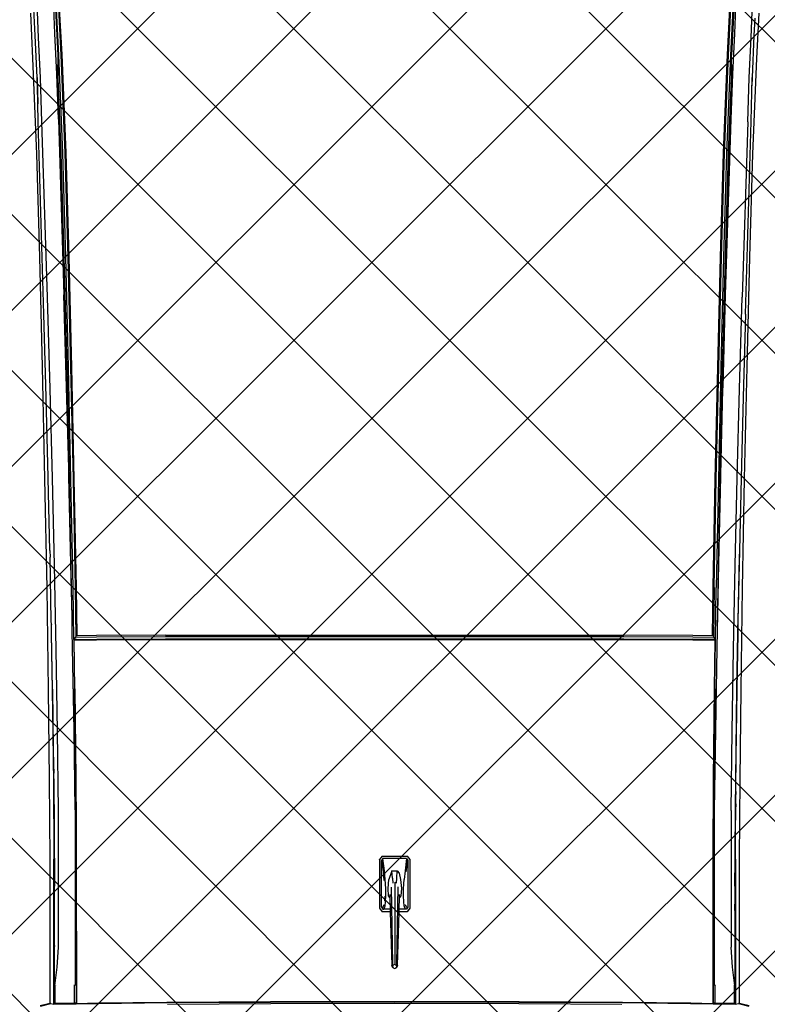
# Model space of a CAD drawing. Units: inches. Extents: x 2167 to 2589, y 1680 to 2489.
# Tile 16 of 38: x 2353 to 2387, y 1727 to 1772. Entities that reach past the tile are written whole.
import ezdxf

# ---------------------------------------------------------------- set-up
doc = ezdxf.new("R2010")
doc.units = ezdxf.units.IN
doc.header["$MEASUREMENT"] = 0
doc.layers.get('0').update_dxf_attribs({"color": 250})
doc.layers.add('C-PRKG-VEHS', color=8, linetype='Continuous', lineweight=13)
doc.layers.add('L-PVMT-PATT', color=252, linetype='Continuous', lineweight=13)
doc.layers.add('Edges', color=250, linetype='Continuous')

# ---------------------------------------------------------------- blocks, each defined once
blk = doc.blocks.new('Nissan Qashqai pl')
at = {"layer": 'Edges'}
for p, q in [((9.5168, 12.4903), (9.4761, 12.4919)), ((9.4782, 12.5024), (9.5503, 12.4987)), ((9.4862, 12.4961), (9.514, 12.4949)), ((9.514, 12.4949), (9.5811, 12.492)), ((9.5812, 12.4874), (9.5168, 12.4903)), ((9.5503, 12.4987), (9.7029, 12.4926)), ((9.651, 12.4906), (9.5811, 12.492)), ((9.5811, 12.492), (9.594, 12.4914)), ((9.6514, 12.4849), (9.5812, 12.4874)), ((9.9583, 12.4812), (9.651, 12.4906)), ((9.7029, 12.4926), (9.8673, 12.4878)), ((9.8673, 12.4878), (10.0423, 12.4835)), ((9.6514, 12.4849), (9.9312, 12.4761)), ((10.0776, 12.4719), (9.9312, 12.4761)), ((9.9583, 12.4812), (10.091, 12.4775)), ((10.0423, 12.4835), (10.2211, 12.4795)), ((10.2201, 12.4683), (10.0776, 12.4719)), ((10.091, 12.4775), (10.2202, 12.4743)), ((10.2202, 12.4743), (10.2203, 12.4743)), ((10.2203, 12.4743), (10.3353, 12.4717)), ((10.2211, 12.4795), (10.3955, 12.4762)), ((10.3353, 12.4717), (10.4477, 12.4694)), ((10.3353, 12.4717), (10.346, 12.4714)), ((10.3955, 12.4762), (10.5572, 12.4737)), ((10.5572, 12.4737), (10.7004, 12.4722)), ((10.7004, 12.4722), (10.8279, 12.4715)), ((11.0575, 12.4714), (11.0581, 12.4738)), ((11.0581, 12.4738), (11.0614, 12.4872)), ((11.0582, 12.47), (11.0624, 12.4866)), ((9.4694, 12.4654), (9.5105, 12.4637)), ((9.4706, 12.4561), (9.5443, 12.4522)), ((9.5446, 12.4542), (9.4709, 12.4581)), ((9.472, 12.463), (9.5454, 12.4591)), ((9.472, 12.4614), (9.5454, 12.4576)), ((9.5105, 12.4637), (9.5755, 12.4608)), ((9.5454, 12.4591), (9.5454, 12.4593)), ((9.5695, 12.4589), (9.5454, 12.4591)), ((9.5454, 12.4576), (9.7014, 12.4513)), ((9.5609, 12.4593), (9.5695, 12.4589)), ((9.5786, 12.4588), (9.5695, 12.4589)), ((9.5695, 12.4589), (9.7014, 12.4536)), ((9.5755, 12.4608), (9.6472, 12.4581)), ((9.6206, 12.4581), (9.5786, 12.4588)), ((9.6714, 12.4567), (9.6206, 12.4581)), ((9.6414, 12.458), (9.6407, 12.458)), ((9.6472, 12.4581), (9.9278, 12.4492)), ((9.6549, 12.4576), (9.6558, 12.4574)), ((9.6825, 12.4564), (9.6714, 12.4567)), ((9.6825, 12.4564), (9.6829, 12.4563)), ((9.6943, 12.456), (9.6825, 12.4564)), ((9.6943, 12.4558), (9.6943, 12.456)), ((9.6951, 12.456), (9.6943, 12.456)), ((9.6951, 12.4558), (9.6951, 12.456)), ((9.8565, 12.451), (9.6951, 12.456)), ((10.3586, 12.4651), (10.2201, 12.4683)), ((10.346, 12.4714), (10.4477, 12.4694)), ((10.4931, 12.4624), (10.3586, 12.4651)), ((10.4477, 12.4694), (10.4538, 12.4693)), ((10.4538, 12.4693), (10.4681, 12.469)), ((10.4676, 12.4691), (10.4538, 12.4693)), ((10.5566, 12.4677), (10.4676, 12.4691)), ((10.4676, 12.4691), (10.546, 12.4677)), ((10.4681, 12.469), (10.5866, 12.467)), ((10.6237, 12.4603), (10.4931, 12.4624)), ((10.546, 12.4677), (10.546, 12.4678)), ((10.546, 12.4677), (10.5576, 12.4675)), ((10.7, 12.4662), (10.5566, 12.4677)), ((10.5576, 12.4675), (10.6649, 12.4659)), ((10.5866, 12.467), (10.6649, 12.4659)), ((10.7502, 12.4586), (10.6237, 12.4603)), ((10.6649, 12.4659), (10.6786, 12.4658)), ((10.6649, 12.4659), (10.6772, 12.4657)), ((10.6786, 12.4657), (10.6772, 12.4657)), ((10.6786, 12.4658), (10.6786, 12.4662)), ((10.6786, 12.4657), (10.6786, 12.4658)), ((10.6786, 12.4658), (10.6801, 12.4657)), ((10.6786, 12.4657), (10.6801, 12.4657)), ((10.6801, 12.4662), (10.6801, 12.4657)), ((10.6801, 12.4657), (10.6801, 12.4657)), ((10.6801, 12.4657), (10.6811, 12.4657)), ((10.6801, 12.4657), (10.6811, 12.4657)), ((10.6811, 12.4662), (10.6811, 12.4657)), ((10.6811, 12.4657), (10.6811, 12.4657)), ((10.6811, 12.4657), (10.6966, 12.4654)), ((10.6811, 12.4657), (10.6991, 12.4655)), ((10.6811, 12.4657), (10.6991, 12.4655)), ((10.6966, 12.4654), (10.7144, 12.4653)), ((10.6991, 12.4655), (10.7144, 12.4653)), ((10.7201, 12.4661), (10.7, 12.4662)), ((10.7144, 12.4653), (10.7239, 12.4653)), ((10.7201, 12.4661), (10.7306, 12.4653)), ((10.7395, 12.4659), (10.7201, 12.4661)), ((10.7239, 12.4653), (10.7248, 12.4653)), ((10.7306, 12.4653), (10.7248, 12.4653)), ((10.7311, 12.4652), (10.7306, 12.4653)), ((10.7495, 12.4652), (10.7311, 12.4652)), ((10.7311, 12.4652), (10.7502, 12.4651)), ((10.7395, 12.4659), (10.7495, 12.4652)), ((10.7923, 12.4656), (10.7395, 12.4659)), ((10.8179, 12.4648), (10.7495, 12.4652)), ((10.7502, 12.4651), (10.7504, 12.4651)), ((10.7502, 12.4586), (10.968, 12.4585)), ((10.7504, 12.4651), (10.7808, 12.4649)), ((10.7808, 12.4649), (10.8179, 12.4648)), ((10.7923, 12.4652), (10.7923, 12.4656)), ((10.7933, 12.4656), (10.7923, 12.4656)), ((10.7933, 12.4652), (10.7933, 12.4656)), ((10.804, 12.4656), (10.7933, 12.4656)), ((10.804, 12.4653), (10.804, 12.4656)), ((10.8075, 12.4655), (10.804, 12.4656)), ((10.8075, 12.4655), (10.8075, 12.4653)), ((10.811, 12.4655), (10.8075, 12.4655)), ((10.811, 12.4655), (10.811, 12.4653)), ((10.8145, 12.4655), (10.811, 12.4655)), ((10.8145, 12.4653), (10.8145, 12.4655)), ((10.8279, 12.4654), (10.8145, 12.4655)), ((10.8277, 12.4647), (10.8179, 12.4648)), ((10.8711, 12.4646), (10.8277, 12.4647)), ((10.8279, 12.4715), (11.0544, 12.4714)), ((10.8279, 12.4654), (11.0592, 12.4653)), ((10.8711, 12.4646), (10.8824, 12.4646)), ((10.8824, 12.4646), (10.8825, 12.4646)), ((10.8825, 12.4646), (10.8884, 12.4646)), ((10.8884, 12.4646), (10.8923, 12.4646)), ((10.8923, 12.4646), (10.8996, 12.4646)), ((10.9097, 12.4646), (10.8996, 12.4646)), ((10.9097, 12.4646), (10.9399, 12.4646)), ((10.9399, 12.4646), (10.9491, 12.4645)), ((10.9491, 12.4645), (11.0301, 12.4645)), ((11, 12.4605), (10.968, 12.4585)), ((11.0301, 12.4645), (11, 12.4605)), ((11.0301, 12.4637), (11.0287, 12.4637)), ((11.03, 12.4635), (11.0301, 12.4637)), ((11.0301, 12.4642), (11.0301, 12.4645)), ((11.0574, 12.4637), (11.0301, 12.4637)), ((11.0544, 12.4714), (11.0575, 12.4714)), ((11.0568, 12.4323), (11.0574, 12.4637)), ((11.0574, 12.4637), (11.0592, 12.4653)), ((11.0575, 12.4714), (11.0582, 12.47)), ((11.0592, 12.4653), (11.0582, 12.47)), ((11.0585, 12.43), (11.0592, 12.4653)), ((9.5443, 12.4522), (9.701, 12.4459)), ((9.7011, 12.4478), (9.5446, 12.4542)), ((9.701, 12.4459), (9.8673, 12.441)), ((9.8673, 12.443), (9.7011, 12.4478)), ((9.7014, 12.4536), (9.8673, 12.4488)), ((9.7014, 12.4513), (9.8673, 12.4464)), ((9.9794, 12.4475), (9.8565, 12.451)), ((9.8673, 12.4488), (10.0429, 12.4444)), ((9.8673, 12.4464), (10.0429, 12.4421)), ((10.043, 12.4387), (9.8673, 12.443)), ((9.8673, 12.441), (10.0431, 12.4367)), ((9.9278, 12.4492), (10.0747, 12.445)), ((10.0998, 12.4443), (9.9794, 12.4475)), ((10.0429, 12.4444), (10.2216, 12.4404)), ((10.0429, 12.4421), (10.2215, 12.4381)), ((10.0747, 12.445), (10.078, 12.4449)), ((10.078, 12.4449), (10.2146, 12.4414)), ((10.2146, 12.4414), (10.0998, 12.4443)), ((10.2146, 12.4414), (10.2175, 12.4413)), ((10.2175, 12.4413), (10.3564, 12.4382)), ((10.2216, 12.4404), (10.3947, 12.4371)), ((10.2218, 12.4347), (10.043, 12.4387)), ((10.0431, 12.4367), (10.2218, 12.4327)), ((10.2215, 12.4381), (10.3945, 12.4348)), ((10.3947, 12.4314), (10.2218, 12.4347)), ((10.2218, 12.4327), (10.3947, 12.4294)), ((10.3564, 12.4382), (10.4638, 12.436)), ((10.4773, 12.4335), (10.3945, 12.4348)), ((10.3947, 12.4371), (10.4638, 12.436)), ((10.3947, 12.4314), (10.4735, 12.4301)), ((10.3947, 12.4294), (10.4715, 12.4282)), ((10.4638, 12.436), (10.4914, 12.4355)), ((10.4715, 12.4282), (10.4711, 12.3973)), ((10.4731, 12.3973), (10.4735, 12.4301)), ((10.4735, 12.4301), (10.4773, 12.4335)), ((10.4773, 12.4296), (10.4769, 12.3968)), ((10.4773, 12.4335), (10.4773, 12.4296)), ((10.4785, 12.433), (10.4773, 12.4335)), ((10.5561, 12.4323), (10.4773, 12.4335)), ((10.4781, 12.3972), (10.4785, 12.433)), ((10.5563, 12.4318), (10.4785, 12.433)), ((10.4914, 12.4355), (10.6223, 12.4333)), ((10.5561, 12.4323), (10.6996, 12.4308)), ((10.6999, 12.4304), (10.5563, 12.4318)), ((10.6223, 12.4333), (10.7493, 12.4316)), ((10.6996, 12.4308), (10.7722, 12.4304)), ((10.827, 12.4297), (10.6999, 12.4304)), ((10.7493, 12.4316), (11.0294, 12.4315)), ((10.7722, 12.4304), (10.7722, 12.4302)), ((10.7722, 12.4304), (10.7889, 12.4303)), ((10.7889, 12.4302), (10.7889, 12.4303)), ((10.7889, 12.4303), (10.7923, 12.4303)), ((10.7923, 12.4302), (10.7923, 12.4303)), ((10.7923, 12.4303), (10.7933, 12.4303)), ((10.7933, 12.4302), (10.7933, 12.4303)), ((10.7933, 12.4303), (10.8267, 12.4301)), ((10.8267, 12.4301), (11.0585, 12.43)), ((10.9133, 12.4296), (10.827, 12.4297)), ((10.9133, 12.4296), (10.9133, 12.4298)), ((10.9137, 12.4296), (10.9133, 12.4296)), ((10.9137, 12.4296), (10.9138, 12.4298)), ((10.9715, 12.4296), (10.9137, 12.4296)), ((10.9715, 12.4299), (10.9715, 12.4296)), ((11.0579, 12.4296), (10.9715, 12.4296)), ((11.0281, 12.4323), (11.0568, 12.4323)), ((11.0294, 12.4315), (11.0294, 12.4316)), ((11.0295, 12.4341), (11.0295, 12.4343)), ((11.0568, 12.4323), (11.0585, 12.43)), ((11.0572, 12.3942), (11.0579, 12.4296)), ((11.0579, 12.3938), (11.0585, 12.43)), ((11.0579, 12.4296), (11.0585, 12.43)), ((10.4711, 12.3973), (10.4706, 12.2875)), ((10.4726, 12.2875), (10.4731, 12.3973)), ((10.4764, 12.2872), (10.4769, 12.3968)), ((10.4776, 12.2874), (10.4781, 12.3972)), ((11.056, 12.2851), (11.0572, 12.3942)), ((11.0566, 12.2849), (11.0579, 12.3938)), ((10.4706, 11.5566), (10.4706, 12.2875)), ((10.4726, 11.5567), (10.4726, 12.2875)), ((10.4764, 11.5569), (10.4764, 12.2872)), ((10.4776, 11.5567), (10.4776, 12.2874)), ((11.0551, 12.1203), (11.056, 12.2851)), ((11.0557, 12.1202), (11.0566, 12.2849)), ((11.0595, 12.2842), (11.0586, 12.1198)), ((11.0547, 11.9221), (11.0551, 12.1203)), ((11.0554, 11.9221), (11.0557, 12.1202)), ((11.0586, 12.1198), (11.0583, 11.9221)), ((10.8228, 11.9421), (10.8224, 11.9421)), ((10.8228, 11.9421), (10.8283, 11.9461)), ((10.8228, 11.9021), (10.8228, 11.9421)), ((10.827, 11.9408), (10.8301, 11.9431)), ((10.827, 11.9408), (10.827, 11.9033)), ((10.827, 11.9408), (10.8467, 11.9386)), ((10.8279, 11.9461), (10.8283, 11.9461)), ((10.8283, 11.9461), (10.906, 11.9461)), ((10.8483, 11.9406), (10.8301, 11.9431)), ((10.8301, 11.9431), (10.9043, 11.9431)), ((10.8467, 11.9386), (10.8603, 11.9373)), ((10.9035, 11.9403), (10.9008, 11.9391)), ((10.9057, 11.9384), (10.9021, 11.9372)), ((10.905, 11.9414), (10.9035, 11.9403)), ((10.9043, 11.9431), (10.9074, 11.9408)), ((10.9043, 11.9431), (10.905, 11.9414)), ((10.9074, 11.9393), (10.9057, 11.9384)), ((10.906, 11.9461), (10.9116, 11.9421)), ((10.9074, 11.9408), (10.9074, 11.9393)), ((10.9074, 11.9393), (10.9074, 11.9291)), ((10.9116, 11.9421), (10.9116, 11.929)), ((10.8467, 11.9263), (10.8501, 11.9295)), ((10.8467, 11.9178), (10.8467, 11.9263)), ((10.8579, 11.9255), (10.8467, 11.9263)), ((10.8501, 11.9295), (10.8603, 11.9316)), ((10.8662, 11.925), (10.8579, 11.9255)), ((10.8746, 11.9363), (10.8603, 11.9373)), ((10.8603, 11.9316), (10.8746, 11.9327)), ((10.8647, 11.9221), (10.996, 11.9221)), ((10.9946, 11.9254), (10.872, 11.9276)), ((10.8861, 11.9361), (10.8746, 11.9363)), ((10.8746, 11.9327), (10.8861, 11.9319)), ((10.889, 11.9296), (10.884, 11.9298)), ((10.8959, 11.9365), (10.8861, 11.9361)), ((10.8861, 11.9319), (10.889, 11.9296)), ((10.9074, 11.9291), (10.889, 11.9296)), ((10.9021, 11.9372), (10.8959, 11.9365)), ((10.9116, 11.929), (10.9074, 11.9291)), ((10.9973, 11.9268), (10.9116, 11.929)), ((10.9969, 11.9247), (10.9946, 11.9254)), ((10.9969, 11.9247), (10.996, 11.9221)), ((10.996, 11.9221), (10.9969, 11.9195)), ((10.999, 11.9258), (10.9969, 11.9247)), ((10.9973, 11.9268), (11.0001, 11.9254)), ((10.999, 11.9258), (10.9973, 11.9268)), ((11.0012, 11.9247), (10.999, 11.9258)), ((11.0012, 11.9247), (11.0001, 11.9254)), ((11.002, 11.9221), (11.0012, 11.9247)), ((11.0012, 11.9195), (11.002, 11.9221)), ((11.0551, 11.7239), (11.0547, 11.9221)), ((11.0557, 11.724), (11.0554, 11.9221)), ((11.0583, 11.9221), (11.0586, 11.7244)), ((10.8579, 11.9187), (10.8467, 11.9178)), ((10.8467, 11.9178), (10.8603, 11.9126)), ((10.8603, 11.9068), (10.8467, 11.9056)), ((10.8579, 11.9187), (10.8662, 11.9191)), ((10.8746, 11.9115), (10.8603, 11.9126)), ((10.8746, 11.9078), (10.8603, 11.9068)), ((10.8723, 11.9165), (10.9946, 11.9187)), ((10.8861, 11.9122), (10.8746, 11.9115)), ((10.8861, 11.908), (10.8746, 11.9078)), ((10.884, 11.9144), (10.889, 11.9145)), ((10.889, 11.9145), (10.8861, 11.9122)), ((10.8959, 11.9077), (10.8861, 11.908)), ((10.8871, 11.9063), (10.8944, 11.906)), ((10.889, 11.9145), (10.9074, 11.915)), ((10.9021, 11.9069), (10.8959, 11.9077)), ((10.9057, 11.9058), (10.9021, 11.9069)), ((10.9074, 11.915), (10.9116, 11.9151)), ((10.9074, 11.915), (10.9074, 11.9049)), ((10.9116, 11.9151), (10.9973, 11.9173)), ((10.9116, 11.9151), (10.9116, 11.9021)), ((10.9946, 11.9187), (10.9969, 11.9195)), ((10.9969, 11.9195), (10.999, 11.9184)), ((11.0001, 11.9187), (10.9973, 11.9173)), ((10.9973, 11.9173), (10.999, 11.9184)), ((10.999, 11.9184), (10.9996, 11.9187)), ((10.9996, 11.9187), (11.0012, 11.9195)), ((11.0001, 11.9187), (10.9996, 11.9187)), ((11.0012, 11.9195), (11.0001, 11.9187)), ((10.8224, 11.9021), (10.8228, 11.9021)), ((10.8228, 11.9021), (10.8283, 11.8981)), ((10.8467, 11.9056), (10.827, 11.9033)), ((10.827, 11.9033), (10.8301, 11.9011)), ((10.8283, 11.8981), (10.8279, 11.8981)), ((10.8283, 11.8981), (10.906, 11.8981)), ((10.8301, 11.9011), (10.8483, 11.9036)), ((10.9043, 11.9011), (10.8301, 11.9011)), ((10.8483, 11.9036), (10.8619, 11.905)), ((10.9008, 11.905), (10.9035, 11.9039)), ((10.9035, 11.9039), (10.905, 11.9028)), ((10.9043, 11.9011), (10.9074, 11.9033)), ((10.905, 11.9028), (10.9043, 11.9011)), ((10.9074, 11.9049), (10.9057, 11.9058)), ((10.906, 11.8981), (10.9116, 11.9021)), ((10.9074, 11.9033), (10.9074, 11.9049)), ((10.9074, 11.9033), (10.9074, 11.9048)), ((11.056, 11.559), (11.0551, 11.7239)), ((11.0566, 11.5593), (11.0557, 11.724)), ((11.0586, 11.7244), (11.0595, 11.5599)), ((10.4706, 11.5566), (10.4711, 11.4469)), ((10.4731, 11.4469), (10.4726, 11.5567)), ((10.4769, 11.4474), (10.4764, 11.5569)), ((10.4781, 11.4469), (10.4776, 11.5567)), ((11.0572, 11.4499), (11.056, 11.559)), ((11.0579, 11.4504), (11.0566, 11.5593)), ((10.4711, 11.4469), (10.4715, 11.416)), ((10.4735, 11.414), (10.4731, 11.4469)), ((10.4773, 11.4146), (10.4769, 11.4474)), ((10.4785, 11.4111), (10.4781, 11.4469)), ((11.0579, 11.4146), (11.0572, 11.4499)), ((11.0585, 11.4142), (11.0579, 11.4504)), ((10.0431, 11.4075), (9.8673, 11.4031)), ((9.8673, 11.4012), (10.043, 11.4055)), ((10.2215, 11.406), (10.0429, 11.4021)), ((10.2216, 11.4037), (10.0429, 11.3998)), ((10.043, 11.4055), (10.2218, 11.4094)), ((10.2218, 11.4114), (10.0431, 11.4075)), ((10.3564, 11.406), (10.2175, 11.4028)), ((10.3945, 11.4094), (10.2215, 11.406)), ((10.3947, 11.4071), (10.2216, 11.4037)), ((10.3947, 11.4148), (10.2218, 11.4114)), ((10.2218, 11.4094), (10.3947, 11.4128)), ((10.4416, 11.4077), (10.3564, 11.406)), ((10.4773, 11.4107), (10.3945, 11.4094)), ((10.4715, 11.416), (10.3947, 11.4148)), ((10.3947, 11.4128), (10.4735, 11.414)), ((10.4416, 11.4078), (10.3947, 11.4071)), ((10.4519, 11.4079), (10.4416, 11.4077)), ((10.4519, 11.4079), (10.4416, 11.4078)), ((10.4416, 11.4077), (10.4416, 11.4078)), ((10.4524, 11.408), (10.4519, 11.4079)), ((10.4519, 11.4079), (10.4519, 11.4079)), ((10.4524, 11.4079), (10.4519, 11.4079)), ((10.4524, 11.4079), (10.4524, 11.408)), ((10.4533, 11.408), (10.4524, 11.408)), ((10.4533, 11.4079), (10.4524, 11.4079)), ((10.4638, 11.4081), (10.4533, 11.4079)), ((10.4638, 11.4081), (10.4533, 11.408)), ((10.4533, 11.4079), (10.4533, 11.408)), ((10.4914, 11.4087), (10.4638, 11.4081)), ((10.4773, 11.4107), (10.4735, 11.414)), ((10.4773, 11.4146), (10.4773, 11.4107)), ((10.4773, 11.4107), (10.5561, 11.4119)), ((10.4773, 11.4107), (10.4785, 11.4111)), ((10.5563, 11.4123), (10.4785, 11.4111)), ((10.6223, 11.4109), (10.4914, 11.4087)), ((10.6996, 11.4134), (10.5561, 11.4119)), ((10.5563, 11.4123), (10.6999, 11.4138)), ((10.7493, 11.4125), (10.6223, 11.4109)), ((10.7722, 11.4138), (10.6996, 11.4134)), ((10.6999, 11.4138), (10.7722, 11.4142)), ((10.7493, 11.4125), (11.0294, 11.4126)), ((10.7722, 11.4142), (10.7889, 11.4143)), ((10.7722, 11.4142), (10.7722, 11.4138)), ((10.7889, 11.4139), (10.7722, 11.4138)), ((10.7889, 11.4139), (10.7889, 11.4143)), ((10.7889, 11.4143), (10.7923, 11.4143)), ((10.7923, 11.4139), (10.7889, 11.4139)), ((10.7923, 11.4139), (10.7923, 11.4143)), ((10.7923, 11.4143), (10.7933, 11.4143)), ((10.7933, 11.4139), (10.7923, 11.4139)), ((10.7933, 11.4143), (10.827, 11.4145)), ((10.7933, 11.4139), (10.7933, 11.4143)), ((10.8267, 11.4141), (10.7933, 11.4139)), ((10.8267, 11.4141), (11.0585, 11.4142)), ((10.827, 11.4145), (11.0579, 11.4146)), ((11.0294, 11.4118), (11.0281, 11.4118)), ((11.0294, 11.4125), (11.0294, 11.4126)), ((11.0295, 11.4116), (11.0294, 11.4118)), ((11.0568, 11.4118), (11.0294, 11.4118)), ((11.0585, 11.4142), (11.0568, 11.4118)), ((11.0574, 11.3804), (11.0568, 11.4118)), ((11.0585, 11.4142), (11.0579, 11.4146)), ((11.0592, 11.3789), (11.0585, 11.4142)), ((9.5443, 11.3919), (9.4706, 11.388)), ((9.4709, 11.3861), (9.5446, 11.39)), ((9.701, 11.3983), (9.5443, 11.3919)), ((9.5446, 11.39), (9.7011, 11.3963)), ((9.7014, 11.3929), (9.5454, 11.3866)), ((9.7014, 11.3906), (9.5695, 11.3853)), ((9.6472, 11.3861), (9.9278, 11.3949)), ((9.6714, 11.3874), (9.8565, 11.3931)), ((9.8673, 11.4031), (9.701, 11.3983)), ((9.7011, 11.3963), (9.8673, 11.4012)), ((9.8673, 11.3977), (9.7014, 11.3929)), ((9.8673, 11.3954), (9.7014, 11.3906)), ((9.8565, 11.3931), (9.9794, 11.3967)), ((10.0429, 11.4021), (9.8673, 11.3977)), ((10.0429, 11.3998), (9.8673, 11.3954)), ((10.0747, 11.3991), (9.9278, 11.3949)), ((9.9794, 11.3967), (10.0965, 11.3998)), ((10.2043, 11.4025), (10.0747, 11.3991)), ((10.0965, 11.3998), (10.0998, 11.3999)), ((10.0998, 11.3999), (10.2043, 11.4025)), ((10.2175, 11.4028), (10.2043, 11.4025)), ((9.5105, 11.3805), (9.4694, 11.3788)), ((9.5454, 11.3866), (9.472, 11.3828)), ((9.472, 11.3812), (9.5454, 11.3851)), ((9.5755, 11.3834), (9.5105, 11.3805)), ((9.5454, 11.3851), (9.5695, 11.3853)), ((9.5454, 11.3848), (9.5454, 11.3851)), ((9.5695, 11.3853), (9.5609, 11.3849)), ((9.5695, 11.3853), (9.5786, 11.3853)), ((9.6472, 11.3861), (9.5755, 11.3834)), ((9.5786, 11.3853), (9.6206, 11.3861)), ((9.6206, 11.3861), (9.6714, 11.3874)), ((9.9312, 11.3681), (10.0776, 11.3722)), ((10.0776, 11.3722), (10.2201, 11.3759)), ((10.2201, 11.3759), (10.3586, 11.3791)), ((10.3353, 11.3725), (10.2203, 11.3699)), ((10.3353, 11.3725), (10.346, 11.3727)), ((10.4477, 11.3747), (10.346, 11.3727)), ((10.3586, 11.3791), (10.4931, 11.3817)), ((10.4537, 11.3749), (10.4477, 11.3747)), ((10.4537, 11.3749), (10.4538, 11.3749)), ((10.4681, 11.3752), (10.4538, 11.3749)), ((10.4676, 11.3751), (10.4538, 11.3749)), ((10.5576, 11.3766), (10.4676, 11.3751)), ((10.5566, 11.3765), (10.4676, 11.3751)), ((10.4676, 11.3751), (10.4676, 11.3751)), ((10.5866, 11.3772), (10.4681, 11.3752)), ((10.4931, 11.3817), (10.6237, 11.3839)), ((10.5566, 11.3765), (10.7, 11.378)), ((10.6649, 11.3783), (10.5576, 11.3766)), ((10.6649, 11.3783), (10.5866, 11.3772)), ((10.6237, 11.3839), (10.7502, 11.3855)), ((10.6908, 11.3785), (10.6649, 11.3783)), ((10.6649, 11.3783), (10.6772, 11.3784)), ((10.6966, 11.3787), (10.6772, 11.3784)), ((10.6772, 11.3784), (10.6908, 11.3785)), ((10.6991, 11.3786), (10.6908, 11.3785)), ((10.7144, 11.3788), (10.6966, 11.3787)), ((10.6999, 11.3786), (10.6991, 11.3786)), ((10.6999, 11.3786), (10.7808, 11.3793)), ((10.7144, 11.3788), (10.6999, 11.3786)), ((10.7, 11.378), (10.8279, 11.3787)), ((10.8279, 11.3727), (10.7004, 11.372)), ((10.7239, 11.3789), (10.7144, 11.3788)), ((10.7248, 11.3789), (10.7239, 11.3789)), ((10.7808, 11.3793), (10.7248, 11.3789)), ((10.7502, 11.3855), (10.968, 11.3857)), ((10.7808, 11.3793), (10.8711, 11.3796)), ((10.9431, 11.3796), (10.8279, 11.3787)), ((10.8279, 11.3787), (11.0552, 11.3789)), ((10.9614, 11.3788), (10.8279, 11.3787)), ((11.0544, 11.3728), (10.8279, 11.3727)), ((10.896, 11.3796), (10.8711, 11.3796)), ((10.9097, 11.3796), (10.896, 11.3796)), ((10.9431, 11.3796), (10.9097, 11.3796)), ((10.9478, 11.3796), (10.9431, 11.3796)), ((10.9491, 11.3796), (10.9478, 11.3796)), ((10.9668, 11.3796), (10.9491, 11.3796)), ((10.9614, 11.3788), (10.9668, 11.3796)), ((10.9711, 11.3788), (10.9614, 11.3788)), ((10.9668, 11.3796), (10.967, 11.3796)), ((10.9765, 11.3796), (10.967, 11.3796)), ((10.968, 11.3857), (11, 11.3837)), ((10.9765, 11.3796), (10.9711, 11.3788)), ((10.9766, 11.3788), (10.9711, 11.3788)), ((10.9765, 11.3796), (10.9766, 11.3788)), ((10.9825, 11.3796), (10.9765, 11.3796)), ((11.0592, 11.3789), (10.9766, 11.3788)), ((11.0301, 11.3796), (10.9825, 11.3796)), ((11, 11.3837), (11.0301, 11.3796)), ((11.0287, 11.3804), (11.0301, 11.3804)), ((11.0301, 11.3803), (11.0292, 11.3802)), ((11.03, 11.3822), (11.03, 11.3824)), ((11.0301, 11.3803), (11.0301, 11.3804)), ((11.0301, 11.3804), (11.0554, 11.3804)), ((11.0554, 11.3804), (11.0301, 11.3803)), ((11.0301, 11.3796), (11.0301, 11.3803)), ((11.0575, 11.3728), (11.0544, 11.3728)), ((11.0554, 11.3804), (11.0574, 11.3804)), ((11.0592, 11.3789), (11.0574, 11.3804)), ((11.0582, 11.3742), (11.0575, 11.3728)), ((11.0581, 11.3704), (11.0575, 11.3728)), ((11.0582, 11.3742), (11.0592, 11.3789)), ((11.0624, 11.3576), (11.0582, 11.3742)), ((9.5168, 11.3539), (9.5812, 11.3568)), ((9.5812, 11.3568), (9.6514, 11.3592)), ((9.9583, 11.363), (9.651, 11.3536)), ((9.6514, 11.3592), (9.9312, 11.3681)), ((10.0423, 11.3607), (9.8673, 11.3563)), ((10.091, 11.3666), (9.9583, 11.363)), ((10.2211, 11.3646), (10.0423, 11.3607)), ((10.2191, 11.3699), (10.091, 11.3666)), ((10.2202, 11.3699), (10.2191, 11.3699)), ((10.2202, 11.3699), (10.2203, 11.3699)), ((10.3955, 11.368), (10.2211, 11.3646)), ((10.5572, 11.3704), (10.3955, 11.368)), ((10.7004, 11.372), (10.5572, 11.3704)), ((11.0614, 11.3569), (11.0581, 11.3704)), ((9.514, 11.3492), (9.4605, 11.3465)), ((9.4761, 11.3522), (9.5168, 11.3539)), ((9.5503, 11.3455), (9.4782, 11.3418)), ((9.5811, 11.3522), (9.514, 11.3492)), ((9.7029, 11.3516), (9.5503, 11.3455)), ((9.5811, 11.3522), (9.6231, 11.3531)), ((9.594, 11.3527), (9.5811, 11.3522)), ((9.6231, 11.3531), (9.594, 11.3527)), ((9.651, 11.3536), (9.6231, 11.3531)), ((9.8673, 11.3563), (9.7029, 11.3516))]:
    blk.add_line(p, q, dxfattribs=at)
blk = doc.blocks.new('car')
blk.add_blockref('Nissan Qashqai pl', (-9.7433, -11.9151))
blk = doc.blocks.new('carr')
blk.add_blockref('car', (0.5124, -0.007))

msp = doc.modelspace()

# ---------------------------------------------------------------- hatches: boundary and pattern name
at = {"layer": 'L-PVMT-PATT'}
h = msp.add_hatch(dxfattribs=at)
h.set_pattern_fill('ANSI37', color=256, scale=40)
h.paths.add_polyline_path([(2417.548, 1783.695), (2417.548, 1846.042), (2239.361, 1846.042), (2239.361, 1687.695), (2369.843, 1687.695), (2369.843, 1696.695), (2375.607, 1696.695), (2416.107, 1696.695), (2417.548, 1696.695)])

# ---------------------------------------------------------------- block references
at = {"layer": 'C-PRKG-VEHS', "xscale": 28.42784210623918, "yscale": 28.42784210623918, "zscale": 28.42784210623918, "rotation": 270}
msp.add_blockref('carr', (2369.852, 1779.037), dxfattribs=at)

doc.saveas('drawing.dxf')
